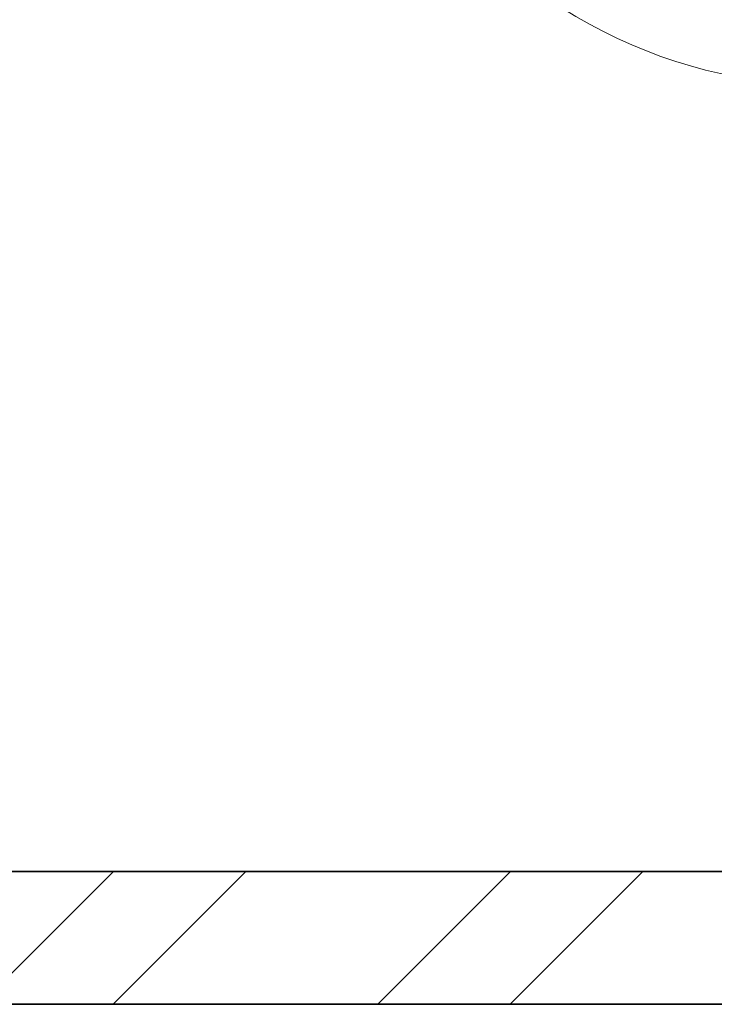
# Model space of a CAD drawing. Units: inches. Extents: x 1885 to 2748, y 783 to 2421.
# Tile 43 of 117: x 2192 to 2216, y 1558 to 1591. Entities that reach past the tile are written whole.
import ezdxf

# ---------------------------------------------------------------- set-up
doc = ezdxf.new("R2010")
doc.units = ezdxf.units.IN
doc.layers.add('A-DOOR', color=31, linetype='Continuous', lineweight=18)
doc.layers.add('A-WALL', color=7, linetype='Continuous', lineweight=35)
doc.layers.add('A-WALL-PATT', color=85, linetype='Continuous', lineweight=13, true_color=0x58ba48)

msp = doc.modelspace()

# ---------------------------------------------------------------- hatches: boundary and pattern name
at = {"layer": 'A-WALL-PATT'}
h = msp.add_hatch(dxfattribs=at)
h.set_pattern_fill('ANSI32', color=256)
h.paths.add_polyline_path([(2007.772, 2318.006), (1980.774, 2318.006), (1980.774, 2281.215), (1985.274, 2281.215), (1985.274, 2313.506), (2007.772, 2313.506), (2007.772, 2315.756)])
h.paths.add_polyline_path([(2094.324, 2318.006), (2067.772, 2318.006), (2067.772, 2313.506), (2094.324, 2313.506), (2094.324, 2315.756)])
h.paths.add_polyline_path([(2131.367, 2315.756), (2131.367, 2318.006), (2131.189, 2318.006), (2112.609, 2318.006), (2112.609, 2313.506), (2117.274, 2313.506), (2117.274, 2255.201), (2121.774, 2255.201), (2121.774, 2313.506), (2131.367, 2313.506)])
h.paths.add_polyline_path([(2190.512, 2318.006), (2155.367, 2318.006), (2155.367, 2313.506), (2169.774, 2313.506), (2169.774, 2229.506), (2121.774, 2229.506), (2121.774, 2233.451), (2119.524, 2233.451), (2117.274, 2233.451), (2117.274, 2201.101), (2121.774, 2201.101), (2121.774, 2225.006), (2169.774, 2225.006), (2169.774, 2165.006), (2306.274, 2165.006), (2306.274, 2066.006), (2310.774, 2066.006), (2344.274, 2066.006), (2486.274, 2066.006), (2486.274, 1886.006), (2483.02, 1886.006), (2483.02, 1881.506), (2486.274, 1881.506), (2486.274, 1880.678), (2490.774, 1880.678), (2490.774, 2070.506), (2344.274, 2070.506), (2310.774, 2070.506), (2310.774, 2165.006), (2310.774, 2173.636), (2308.524, 2173.636), (2306.274, 2173.636), (2306.274, 2169.506), (2174.274, 2169.506), (2174.274, 2313.506), (2190.512, 2313.506), (2190.512, 2315.756)])
h.paths.add_polyline_path([(1985.274, 2221.215), (1980.774, 2221.215), (1980.774, 2165.006), (1992.774, 2165.006), (1992.774, 2141.927), (1997.274, 2141.927), (1997.274, 2165.006), (2117.274, 2165.006), (2117.274, 2163.126), (2121.774, 2163.126), (2121.774, 2172.734), (2119.524, 2172.734), (2117.274, 2172.734), (2117.274, 2169.506), (1985.274, 2169.506)])
h.paths.add_polyline_path([(1997.274, 2105.927), (1992.774, 2105.927), (1992.774, 2070.506), (2016.774, 2070.506), (2016.774, 2059.123), (2019.024, 2059.123), (2021.274, 2059.123), (2021.274, 2070.506), (2117.274, 2070.506), (2117.274, 2022.506), (2114.423, 2022.506), (2114.423, 2018.006), (2123.627, 2018.006), (2123.627, 2020.256), (2123.627, 2022.506), (2121.774, 2022.506), (2121.774, 2142.587), (2119.524, 2142.587), (2117.274, 2142.587), (2117.274, 2075.006), (1997.274, 2075.006)])
h.paths.add_polyline_path([(2092.029, 2020.256), (2092.029, 2022.506), (2021.274, 2022.506), (2021.274, 2035.123), (2016.774, 2035.123), (2016.774, 2018.006), (2016.774, 1978.784), (2021.274, 1978.784), (2021.274, 2018.006), (2092.029, 2018.006)])
h.paths.add_polyline_path([(2260.938, 2022.506), (2153.105, 2022.506), (2153.105, 2020.256), (2153.105, 2018.006), (2155.274, 2018.006), (2155.274, 1886.006), (2107.629, 1886.006), (2107.629, 1881.506), (2182.911, 1881.506), (2182.911, 1883.756), (2182.911, 1886.006), (2159.774, 1886.006), (2159.774, 2018.006), (2260.938, 2018.006), (2260.938, 2020.256)])
h.paths.add_polyline_path([(2047.629, 1883.756), (2047.629, 1886.006), (2021.274, 1886.006), (2021.274, 1918.784), (2019.024, 1918.784), (2016.774, 1918.784), (2016.774, 1881.506), (2047.629, 1881.506)])
h.paths.add_polyline_path([(2306.361, 1883.756), (2306.361, 1886.006), (2296.274, 1886.006), (2296.274, 1982.006), (2316.535, 1982.006), (2316.535, 1984.256), (2316.535, 1986.506), (2296.274, 1986.506), (2296.274, 2022.506), (2289.276, 2022.506), (2289.276, 2018.006), (2291.774, 2018.006), (2291.774, 1886.006), (2242.911, 1886.006), (2242.911, 1881.506), (2306.361, 1881.506)], flags=17)
h.paths.add_polyline_path([(1985.274, 1843.006), (2021.6, 1843.006), (2021.534, 1845.441), (2021.477, 1847.506), (1980.774, 1847.506), (1980.774, 1809.446), (1985.274, 1809.446)])
h.paths.add_polyline_path([(2131.482, 1845.256), (2131.482, 1847.506), (2081.534, 1847.506), (2081.534, 1843.006), (2117.274, 1843.006), (2117.274, 1784.147), (2119.524, 1784.147), (2121.774, 1784.147), (2121.774, 1843.006), (2131.482, 1843.006)])
h.paths.add_polyline_path([(2203.886, 1847.506), (2155.482, 1847.506), (2155.482, 1843.006), (2169.774, 1843.006), (2169.774, 1759.006), (2121.774, 1759.006), (2121.774, 1761.457), (2117.274, 1761.457), (2117.274, 1730.429), (2121.774, 1730.429), (2121.774, 1754.506), (2177.421, 1754.506), (2177.421, 1756.756), (2177.421, 1759.006), (2174.274, 1759.006), (2174.274, 1843.006), (2203.886, 1843.006)])
h.paths.add_polyline_path([(2335.554, 1845.256), (2335.554, 1847.506), (2239.886, 1847.506), (2239.886, 1843.006), (2306.274, 1843.006), (2306.274, 1759.006), (2199.486, 1759.006), (2199.486, 1754.506), (2310.774, 1754.506), (2310.774, 1843.006), (2335.554, 1843.006)])
h.paths.add_polyline_path([(2348.774, 2022.506), (2344.274, 2022.506), (2344.274, 1986.506), (2341.681, 1986.506), (2341.681, 1982.006), (2344.274, 1982.006), (2344.274, 1886.006), (2330.361, 1886.006), (2330.361, 1881.506), (2361.627, 1881.506), (2361.627, 1883.756), (2361.627, 1886.006), (2348.774, 1886.006)], flags=17)
h.paths.add_polyline_path([(2283.251, 2315.756), (2283.251, 2318.006), (2238.512, 2318.006), (2238.512, 2313.506), (2283.251, 2313.506)], flags=17)
h.paths.add_polyline_path([(2363.274, 2348.006), (2388.677, 2348.006), (2388.677, 2350.256), (2388.677, 2352.506), (2358.774, 2352.506), (2358.774, 2348.006), (2358.774, 2318.006), (2344.481, 2318.006), (2344.481, 2313.506), (2358.774, 2313.506), (2358.774, 2229.506), (2310.774, 2229.506), (2310.774, 2231.952), (2306.274, 2231.952), (2306.274, 2205.611), (2310.774, 2205.611), (2310.774, 2225.006), (2358.774, 2225.006), (2358.774, 2211.506), (2452.329, 2211.506), (2452.329, 2213.756), (2452.329, 2216.006), (2363.274, 2216.006), (2363.274, 2318.006)])
h.paths.add_polyline_path([(2310.774, 2313.506), (2320.481, 2313.506), (2320.481, 2315.756), (2320.481, 2318.006), (2302.728, 2318.006), (2302.728, 2313.506), (2306.274, 2313.506), (2306.274, 2251.076), (2310.774, 2251.076)], flags=17)
h.paths.add_polyline_path([(2490.774, 2352.506), (2486.274, 2352.506), (2448.677, 2352.506), (2448.677, 2348.006), (2486.274, 2348.006), (2486.274, 2318.006), (2486.274, 2216.006), (2481.78, 2216.006), (2481.78, 2211.506), (2486.274, 2211.506), (2486.274, 2165.006), (2493.289, 2165.006), (2493.289, 2167.256), (2493.289, 2169.506), (2490.774, 2169.506), (2490.774, 2313.506), (2494.429, 2313.506), (2494.429, 2318.006), (2490.774, 2318.006)])
h.paths.add_polyline_path([(2534.653, 2318.006), (2515.691, 2318.006), (2515.691, 2313.506), (2534.653, 2313.506), (2534.653, 2315.756)])
h.paths.add_polyline_path([(2618.274, 2318.006), (2594.653, 2318.006), (2594.653, 2313.506), (2613.774, 2313.506), (2613.774, 2281.706), (2618.274, 2281.706)])
h.paths.add_polyline_path([(2618.274, 2221.706), (2613.774, 2221.706), (2613.774, 2169.506), (2554.019, 2169.506), (2554.019, 2165.006), (2613.774, 2165.006), (2613.774, 2152.878), (2618.274, 2152.878)])
h.paths.add_polyline_path([(2618.274, 2128.878), (2616.024, 2128.878), (2613.774, 2128.878), (2613.774, 2117.006), (2529.774, 2117.006), (2529.774, 2165.006), (2532.848, 2165.006), (2532.848, 2169.506), (2522.867, 2169.506), (2522.867, 2165.006), (2525.274, 2165.006), (2525.274, 2117.006), (2525.274, 2112.506), (2525.274, 2108.576), (2529.774, 2108.576), (2529.774, 2112.506), (2613.774, 2112.506), (2613.774, 2080.19), (2618.274, 2080.19)])
h.paths.add_polyline_path([(2618.274, 2044.19), (2616.024, 2044.19), (2613.774, 2044.19), (2613.774, 2015.506), (2529.774, 2015.506), (2529.774, 2088.582), (2527.524, 2088.582), (2525.274, 2088.582), (2525.274, 2011.006), (2613.774, 2011.006), (2613.774, 1956.755), (2618.274, 1956.755)])
h.paths.add_polyline_path([(2618.274, 1881.506), (2618.274, 1896.755), (2613.774, 1896.755), (2613.774, 1881.506), (2613.774, 1847.506), (2592.715, 1847.506), (2592.715, 1843.006), (2613.774, 1843.006), (2613.774, 1765.006), (2613.774, 1760.506), (2609.621, 1760.506), (2609.621, 1756.006), (2613.774, 1756.006), (2613.774, 1660.006), (2608.544, 1660.006), (2608.544, 1655.506), (2613.774, 1655.506), (2613.774, 1508.158), (2618.274, 1508.158)])
h.paths.add_polyline_path([(2565.774, 1843.006), (2568.997, 1843.006), (2568.997, 1847.506), (2490.774, 1847.506), (2490.774, 1849.7), (2488.524, 1849.7), (2486.274, 1849.7), (2486.274, 1847.506), (2477.274, 1847.506), (2477.274, 1838.506), (2477.274, 1821.493), (2486.274, 1821.493), (2486.274, 1838.506), (2561.274, 1838.506), (2561.274, 1765.006), (2486.274, 1765.006), (2486.274, 1786.157), (2477.274, 1786.157), (2477.274, 1765.006), (2477.274, 1756.006), (2486.274, 1756.006), (2565.774, 1756.006), (2585.621, 1756.006), (2585.621, 1758.256), (2585.621, 1760.506), (2565.774, 1760.506), (2565.774, 1765.006)])
h.paths.add_polyline_path([(2486.274, 1651.006), (2561.274, 1651.006), (2561.274, 1567.006), (2486.274, 1567.006), (2486.274, 1591.321), (2477.274, 1591.321), (2477.274, 1567.006), (2477.274, 1558.006), (2477.274, 1555.439), (2481.774, 1555.439), (2481.774, 1558.006), (2568.653, 1558.006), (2568.653, 1560.256), (2568.653, 1562.506), (2565.774, 1562.506), (2565.774, 1655.506), (2584.544, 1655.506), (2584.544, 1657.756), (2584.544, 1660.006), (2565.774, 1660.006), (2486.274, 1660.006), (2477.274, 1660.006), (2477.274, 1651.006), (2477.274, 1632.989), (2486.274, 1632.989)])
h.paths.add_polyline_path([(2449.967, 1883.756), (2449.967, 1886.006), (2421.627, 1886.006), (2421.627, 1881.506), (2449.967, 1881.506)], flags=17)
h.paths.add_polyline_path([(2447.274, 1847.506), (2395.554, 1847.506), (2395.554, 1843.006), (2442.774, 1843.006), (2442.774, 1809.27), (2447.274, 1809.27)])
h.paths.add_polyline_path([(1985.274, 1749.446), (1980.774, 1749.446), (1980.774, 1694.504), (1985.274, 1694.504), (1985.274, 1694.506), (1986.897, 1694.506), (1986.897, 1697.78), (1986.897, 1699.006), (1985.274, 1699.006)])
h.paths.add_polyline_path([(2152.774, 1699.006), (2121.774, 1699.006), (2121.774, 1703.668), (2119.524, 1703.668), (2117.274, 1703.668), (2117.274, 1699.006), (2009.219, 1699.006), (2009.219, 1694.506), (2148.274, 1694.506), (2148.274, 1692.631), (2152.774, 1692.631)])
h.paths.add_polyline_path([(2016.274, 1694.506), (2011.774, 1694.506), (2011.774, 1558.006), (2040.806, 1558.006), (2040.806, 1560.256), (2040.806, 1562.506), (2016.274, 1562.506)])
h.paths.add_polyline_path([(2152.774, 1663.017), (2150.524, 1663.017), (2148.274, 1663.017), (2148.274, 1562.506), (2100.806, 1562.506), (2100.806, 1558.006), (2165.119, 1558.006), (2165.119, 1560.256), (2165.119, 1562.506), (2152.774, 1562.506), (2152.774, 1610.506), (2224.774, 1610.506), (2224.774, 1607.99), (2229.274, 1607.99), (2229.274, 1615.006), (2152.774, 1615.006)])
h.paths.add_polyline_path([(2238.613, 1560.256), (2238.613, 1562.506), (2229.274, 1562.506), (2229.274, 1588.756), (2227.024, 1588.763), (2224.774, 1588.771), (2224.774, 1562.506), (2189.119, 1562.506), (2189.119, 1558.006), (2238.613, 1558.006)])
h.paths.add_polyline_path([(2336.024, 1560.256), (2336.024, 1562.506), (2310.774, 1562.506), (2310.774, 1656.347), (2308.524, 1656.347), (2306.274, 1656.347), (2306.274, 1562.506), (2286.613, 1562.506), (2286.613, 1558.006), (2336.024, 1558.006)])
h.paths.add_polyline_path([(2447.274, 1690.968), (2445.024, 1690.968), (2442.774, 1690.968), (2442.774, 1687.006), (2306.274, 1687.006), (2306.274, 1680.75), (2310.774, 1680.75), (2310.774, 1682.506), (2442.774, 1682.506), (2442.774, 1562.506), (2396.024, 1562.506), (2396.024, 1558.006), (2447.274, 1558.006)])
h.paths.add_polyline_path([(2447.274, 1749.27), (2445.024, 1749.27), (2442.774, 1749.27), (2442.774, 1717.232), (2447.274, 1717.232)])
h.paths.add_polyline_path([(2044.674, 1521.756), (2044.674, 1524.006), (2007.274, 1524.006), (2007.274, 1503.49), (2009.524, 1503.49), (2011.774, 1503.49), (2011.774, 1519.506), (2044.674, 1519.506)])
h.paths.add_polyline_path([(2177.969, 1521.756), (2177.969, 1524.006), (2104.674, 1524.006), (2104.674, 1519.506), (2145.774, 1519.506), (2145.774, 1387.506), (2143.37, 1387.506), (2143.37, 1383.006), (2251.585, 1383.006), (2251.585, 1385.256), (2251.585, 1387.506), (2150.274, 1387.506), (2150.274, 1519.506), (2177.969, 1519.506)])
h.paths.add_polyline_path([(2298.704, 1524.006), (2237.969, 1524.006), (2237.969, 1519.506), (2282.274, 1519.506), (2282.274, 1387.506), (2279.683, 1387.506), (2279.683, 1383.006), (2286.774, 1383.006), (2286.774, 1419.006), (2312.451, 1419.006), (2312.451, 1421.256), (2312.451, 1423.506), (2286.774, 1423.506), (2286.774, 1519.506), (2298.704, 1519.506), (2298.704, 1521.722)], flags=17)
h.paths.add_polyline_path([(2361.897, 1521.756), (2361.897, 1524.006), (2322.704, 1524.006), (2322.704, 1519.506), (2334.774, 1519.506), (2334.774, 1423.506), (2331.93, 1423.506), (2331.93, 1419.006), (2334.774, 1419.006), (2334.774, 1387.506), (2334.774, 1383.228), (2339.274, 1383.228), (2339.274, 1387.506), (2339.274, 1519.506), (2361.897, 1519.506)], flags=17)
h.paths.add_polyline_path([(2447.274, 1521.756), (2447.274, 1524.006), (2421.897, 1524.006), (2421.897, 1519.506), (2447.274, 1519.506)], flags=17)
h.paths.add_polyline_path([(2481.774, 1529.6), (2479.524, 1529.6), (2477.274, 1529.6), (2477.274, 1524.006), (2474.489, 1524.006), (2474.489, 1519.506), (2477.274, 1519.506), (2477.274, 1334.506), (2296.774, 1334.506), (2296.774, 1240.506), (2160.274, 1240.506), (2160.274, 1180.506), (2112.274, 1180.506), (2112.274, 1207.692), (2110.024, 1207.692), (2107.774, 1207.692), (2107.774, 1171.609), (2112.274, 1171.609), (2112.274, 1176.006), (2160.274, 1176.006), (2160.274, 1092.006), (2144.221, 1092.006), (2144.221, 1087.506), (2189.497, 1087.506), (2189.497, 1089.756), (2189.497, 1092.006), (2164.774, 1092.006), (2164.774, 1236.006), (2296.774, 1236.006), (2296.774, 1231.912), (2301.274, 1231.912), (2301.274, 1330.006), (2481.774, 1330.006), (2481.774, 1387.506)])
h.paths.add_polyline_path([(2618.274, 1448.158), (2613.774, 1448.158), (2613.774, 1382.506), (2529.774, 1382.506), (2525.274, 1382.506), (2525.274, 1307.062), (2529.774, 1307.062), (2529.774, 1378.006), (2613.774, 1378.006), (2613.774, 1354.988), (2618.274, 1354.988)])
h.paths.add_polyline_path([(2618.274, 1318.988), (2613.774, 1318.988), (2613.774, 1281.006), (2529.774, 1281.006), (2529.774, 1283.786), (2527.524, 1283.786), (2525.274, 1283.786), (2525.274, 1228.506), (2516.794, 1228.506), (2516.794, 1224.006), (2533.484, 1224.006), (2533.484, 1226.256), (2533.484, 1228.506), (2529.774, 1228.506), (2529.774, 1276.506), (2613.774, 1276.506), (2613.774, 1266.02), (2618.274, 1266.02)])
h.paths.add_polyline_path([(2618.274, 1134.964), (2613.774, 1134.964), (2613.774, 1092.006), (2594.545, 1092.006), (2594.545, 1087.506), (2618.274, 1087.506)])
h.paths.add_polyline_path([(2534.545, 1092.006), (2509.765, 1092.006), (2509.765, 1087.506), (2534.545, 1087.506), (2534.545, 1089.756)])
h.paths.add_polyline_path([(2481.274, 1224.006), (2484.117, 1224.006), (2484.117, 1226.256), (2484.117, 1228.506), (2476.774, 1228.506), (2476.774, 1198.506), (2471.61, 1198.506), (2471.61, 1194.006), (2476.774, 1194.006), (2476.774, 1062.006), (2436.894, 1062.006), (2436.894, 1057.506), (2476.774, 1057.506), (2481.274, 1057.506), (2481.274, 1062.006), (2481.274, 1087.506), (2485.354, 1087.506), (2485.354, 1089.756), (2485.354, 1092.006), (2481.274, 1092.006), (2481.274, 1117.506)])
h.paths.add_polyline_path([(2439.898, 1198.506), (2349.274, 1198.506), (2349.274, 1194.006), (2349.274, 1180.506), (2301.274, 1180.506), (2301.274, 1201.896), (2299.024, 1201.896), (2296.774, 1201.896), (2296.774, 1172.335), (2299.024, 1172.335), (2301.274, 1172.335), (2301.274, 1176.006), (2349.274, 1176.006), (2349.274, 1092.006), (2334.452, 1092.006), (2334.452, 1087.506), (2349.274, 1087.506), (2349.274, 1057.506), (2353.774, 1057.506), (2376.894, 1057.506), (2376.894, 1059.756), (2376.894, 1062.006), (2353.774, 1062.006), (2353.774, 1087.506), (2353.774, 1180.506), (2353.774, 1194.006), (2439.898, 1194.006), (2439.898, 1196.256)])
h.paths.add_polyline_path([(2270.596, 1089.756), (2270.596, 1092.006), (2249.497, 1092.006), (2249.497, 1087.506), (2270.596, 1087.506)], flags=17)
h.paths.add_polyline_path([(2310.452, 1092.006), (2301.274, 1092.006), (2301.274, 1153.292), (2296.774, 1153.292), (2296.774, 1092.006), (2293.786, 1092.006), (2293.786, 1087.506), (2310.452, 1087.506), (2310.452, 1089.756)], flags=17)
h.paths.add_polyline_path([(2112.274, 1150.328), (2110.024, 1150.328), (2107.774, 1150.328), (2107.774, 1092.006), (2104.465, 1092.006), (2104.465, 1087.506), (2120.221, 1087.506), (2120.221, 1089.756), (2120.221, 1092.006), (2112.274, 1092.006)])
h.paths.add_polyline_path([(2082.172, 1092.006), (2058.144, 1092.006), (2058.144, 1087.506), (2082.172, 1087.506), (2082.172, 1089.756)])
h.paths.add_polyline_path([(1975.774, 1145.638), (1971.274, 1145.638), (1971.274, 1087.506), (1980.774, 1087.506), (1998.144, 1087.506), (1998.144, 1089.756), (1998.144, 1092.006), (1985.274, 1092.006), (1975.774, 1092.006)])
h.paths.add_polyline_path([(2112.274, 1244.385), (2110.024, 1244.385), (2107.774, 1244.385), (2107.774, 1240.506), (1992.274, 1240.506), (1992.274, 1271.008), (1987.774, 1271.008), (1987.774, 1240.506), (1980.774, 1240.506), (1975.774, 1240.506), (1971.274, 1240.506), (1971.274, 1205.638), (1975.774, 1205.638), (1975.774, 1236.006), (2107.774, 1236.006), (2107.774, 1233.444), (2112.274, 1233.444), (2112.274, 1236.006)])
h.paths.add_polyline_path([(2112.274, 1383.006), (2114.783, 1383.006), (2114.783, 1385.256), (2114.783, 1387.506), (2102.476, 1387.506), (2102.476, 1383.006), (2107.774, 1383.006), (2107.774, 1335.006), (2011.774, 1335.006), (2011.774, 1349.939), (2007.274, 1349.939), (2007.274, 1335.006), (1987.774, 1335.006), (1987.774, 1330.506), (1987.774, 1307.008), (1992.274, 1307.008), (1992.274, 1330.506), (2007.274, 1330.506), (2107.774, 1330.506), (2107.774, 1264.711), (2112.274, 1264.711)])
h.paths.add_polyline_path([(2077.857, 1387.506), (2011.774, 1387.506), (2011.774, 1390.036), (2009.524, 1390.036), (2007.274, 1390.036), (2007.274, 1373.939), (2011.774, 1373.939), (2011.774, 1383.006), (2077.857, 1383.006)])
h.paths.add_polyline_path([(2011.774, 1443.49), (2007.274, 1443.49), (2007.274, 1410.248), (2011.774, 1410.248)])

# ---------------------------------------------------------------- linework, layer by layer
at = {"layer": 'A-DOOR'}
msp.add_arc((2219.854, 1605.99), 16.83, 180, 295.2133, dxfattribs=at)
at = {"layer": 'A-WALL'}
for p, q in [((2189.119, 1562.506), (2224.774, 1562.506)), ((2189.119, 1558.006), (2238.613, 1558.006))]:
    msp.add_line(p, q, dxfattribs=at)

doc.saveas('drawing.dxf')
